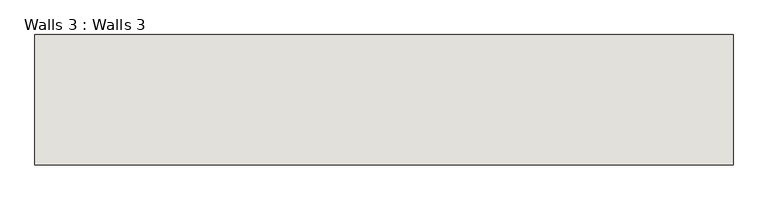
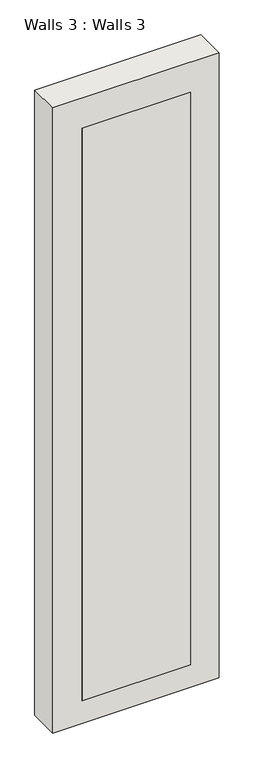
"""IFC4 building model written with IfcOpenShell, lengths in millimetres: wall geometry, Walls 3 : Walls 3."""

from ifc_helpers import new_model, si_unit, frame, origin, place, context, project, spatial, polyline, outline, extrude, source, transform, mapped, element, save


def walls_3_walls_3_7c260857(model_context):
    return source(origin(), model_context, "Body", "SweptSolid", [
        extrude(outline(polyline([(-5888.0442755, 3201.7419215), (-6954.8442755, 3201.7419215), (-6954.8442755, 3506.5419215), (-5888.0442755, 3506.5419215), (-5888.0442755, 3201.7419215)])), frame((0.0, 0.0, 3977.534498), z_axis=(0.0, 0.0, 1.0), x_axis=(1.0, 0.0, 0.0)), (0.0, 0.0, 1.0), 5943.6),
        extrude(outline(polyline([(-5606.7936733, 3201.7419215), (-7242.5350326, 3201.7419215), (-7242.5350326, 3506.5419215), (-5606.7936733, 3506.5419215), (-5606.7936733, 3201.7419215)])), frame((0.0, 0.0, 3741.2191762), z_axis=(0.0, 0.0, 1.0), x_axis=(1.0, 0.0, 0.0)), (0.0, 0.0, 1.0), 6494.582187),
    ])


if __name__ == "__main__":
    model = new_model("IFC4")
    model_context = context("Model", 3, world=origin())
    ifc_project = project(units=[si_unit("LENGTHUNIT", "METRE", prefix="MILLI")], contexts=[model_context])
    site = spatial("IfcSite", under=ifc_project)
    building = spatial("IfcBuilding", under=site)
    placement = place(None, origin())
    walls_3_walls_3_shape = walls_3_walls_3_7c260857(model_context)
    element("IfcWall", 1, ObjectType="Walls 3 : Walls 3", at=placement, inside=building, context=model_context, shape_type="MappedRepresentation", body=[
        mapped(walls_3_walls_3_shape, transform((0.0, 0.0, 0.0), x_axis=(1.0, 0.0, 0.0), y_axis=(0.0, 1.0, 0.0), z_axis=(0.0, 0.0, 1.0))),
    ])
    save(model, "model.ifc")

# Revit data of these elements
# Element 1 (IfcWall, "Walls 3 : Walls 3")
#   Materials on its faces: "Default Wall"
# Materials
#   "Default Wall": colour RGB 128 128 128, transparency 0
